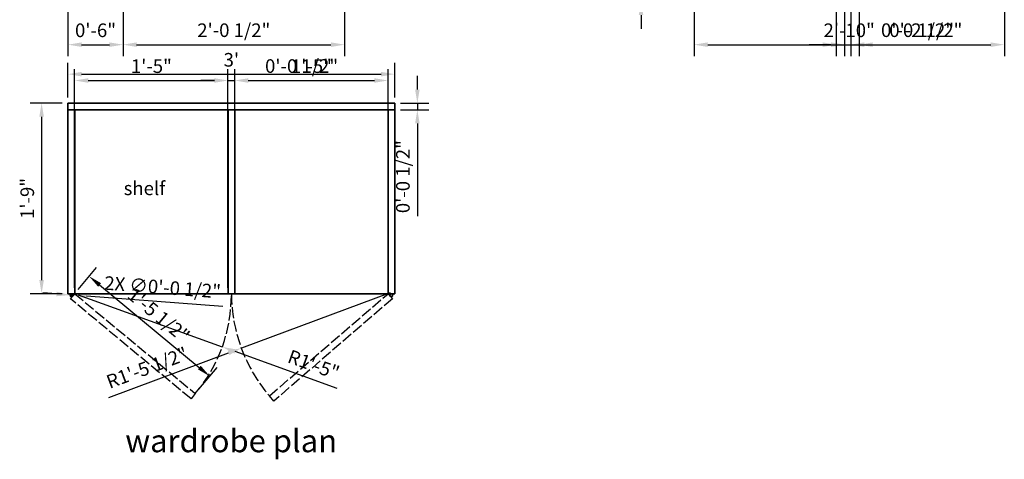
# Model space of a CAD drawing. Units: inches. Extents: x 1145 to 1264, y 2632 to 2775.
# Tile 1 of 2: x 1149 to 1257, y 2632 to 2681. Entities that reach past the tile are written whole.
import ezdxf

# ---------------------------------------------------------------- set-up
doc = ezdxf.new("R2010")
doc.units = ezdxf.units.IN
doc.linetypes.add('ACAD_ISO02W100', pattern=[15, 12, -3])
for name, color, linetype, lineweight in [('A-ANNO-DIMS', 2, 'Continuous', 18), ('A-ANNO-TEXT', 3, 'Continuous', 25), ('A-DOOR', 4, 'ACAD_ISO02W100', 25), ('A-FURN', 7, 'Continuous', 35)]:
    doc.layers.add(name, color=color, linetype=linetype, lineweight=lineweight)
doc.styles.get("Standard").update_dxf_attribs({"font": 'arial.ttf'})
doc.dimstyles.new('ISO-25', dxfattribs={"dimtxt": 1.5, "dimasz": 1.5, "dimexe": 1.25, "dimexo": 0.625, "dimtad": 1, "dimlunit": 3, "dimtxsty": 'Standard', "dimcen": 2.5, "dimadec": 0, "dimazin": 0, "dimtfac": 1, "dimtmove": 0, "dimatfit": 3, "dimfxl": 1, "dimarcsym": 0})

# ---------------------------------------------------------------- blocks, each defined once
blk = doc.blocks.new('*D1')
at = {"layer": 'A-ANNO-DIMS', "color": 0, "lineweight": -2, "transparency": 16777216}
for p, q in [((1153.92, 2671.95), (1153.92, 2675.76)), ((1189.92, 2671.95), (1189.92, 2675.76)), ((1155.42, 2674.51), (1188.42, 2674.51))]:
    blk.add_line(p, q, dxfattribs=at)
at = {"layer": 'A-ANNO-DIMS', "color": 0, "lineweight": 100, "transparency": 16777216}
for points in [[(1155.42, 2674.76), (1155.42, 2674.26), (1153.92, 2674.51)], [(1188.42, 2674.76), (1188.42, 2674.26), (1189.92, 2674.51)]]:
    blk.add_solid(points, dxfattribs=at)
at = {"layer": 'Defpoints', "color": 0, "lineweight": 100, "transparency": 16777216}
for p in [(1189.92, 2674.51), (1153.92, 2671.32), (1189.92, 2671.32)]:
    blk.add_point(p, dxfattribs=at)
at = {"layer": 'A-ANNO-DIMS', "color": 0, "transparency": 16777216, "insert": (1171.92, 2675.9), "char_height": 1.5, "attachment_point": 5}
blk.add_mtext("3'", dxfattribs=at)
blk = doc.blocks.new('*D2')
at = {"layer": 'A-ANNO-DIMS', "color": 0, "lineweight": -2, "transparency": 16777216}
for p, q in [((1153.3, 2671.32), (1149.77, 2671.32)), ((1151.02, 2669.82), (1151.02, 2651.82)), ((1153.3, 2650.32), (1149.77, 2650.32))]:
    blk.add_line(p, q, dxfattribs=at)
at = {"layer": 'A-ANNO-DIMS', "color": 0, "lineweight": 100, "transparency": 16777216}
for points in [[(1150.77, 2669.82), (1151.27, 2669.82), (1151.02, 2671.32)], [(1150.77, 2651.82), (1151.27, 2651.82), (1151.02, 2650.32)]]:
    blk.add_solid(points, dxfattribs=at)
at = {"layer": 'Defpoints', "color": 0, "lineweight": 100, "transparency": 16777216}
for p in [(1153.92, 2671.32), (1151.02, 2650.32), (1153.92, 2650.32)]:
    blk.add_point(p, dxfattribs=at)
at = {"layer": 'A-ANNO-DIMS', "color": 0, "transparency": 16777216, "insert": (1149.63, 2660.82), "char_height": 1.5, "attachment_point": 5, "rotation": 90}
blk.add_mtext('1\'-9"', dxfattribs=at)
blk = doc.blocks.new('*D21')
at = {"layer": 'A-ANNO-DIMS', "color": 0, "lineweight": -2, "transparency": 16777216}
for p, q in [((1153.92, 2681.89), (1153.92, 2676.51)), ((1159.99, 2682.21), (1159.99, 2676.51)), ((1155.42, 2677.76), (1158.49, 2677.76))]:
    blk.add_line(p, q, dxfattribs=at)
at = {"layer": 'A-ANNO-DIMS', "color": 0, "lineweight": 100, "transparency": 16777216}
for points in [[(1155.42, 2678.01), (1155.42, 2677.51), (1153.92, 2677.76)], [(1158.49, 2678.01), (1158.49, 2677.51), (1159.99, 2677.76)]]:
    blk.add_solid(points, dxfattribs=at)
at = {"layer": 'Defpoints', "color": 0, "lineweight": 100, "transparency": 16777216}
for p in [(1153.92, 2682.52), (1159.99, 2682.84), (1159.99, 2677.76)]:
    blk.add_point(p, dxfattribs=at)
at = {"layer": 'A-ANNO-DIMS', "color": 0, "transparency": 16777216, "insert": (1156.96, 2679.15), "char_height": 1.5, "attachment_point": 5}
blk.add_mtext('0\'-6"', dxfattribs=at)
blk = doc.blocks.new('*D22')
at = {"layer": 'A-ANNO-DIMS', "color": 0, "lineweight": -2, "transparency": 16777216}
for p, q in [((1159.99, 2682.21), (1159.99, 2676.51)), ((1184.39, 2682.21), (1184.39, 2676.51)), ((1161.49, 2677.76), (1182.89, 2677.76))]:
    blk.add_line(p, q, dxfattribs=at)
at = {"layer": 'A-ANNO-DIMS', "color": 0, "lineweight": 100, "transparency": 16777216}
for points in [[(1161.49, 2678.01), (1161.49, 2677.51), (1159.99, 2677.76)], [(1182.89, 2678.01), (1182.89, 2677.51), (1184.39, 2677.76)]]:
    blk.add_solid(points, dxfattribs=at)
at = {"layer": 'Defpoints', "color": 0, "lineweight": 100, "transparency": 16777216}
for p in [(1159.99, 2682.84), (1184.39, 2682.84), (1184.39, 2677.76)]:
    blk.add_point(p, dxfattribs=at)
at = {"layer": 'A-ANNO-DIMS', "color": 0, "transparency": 16777216, "insert": (1172.19, 2679.16), "char_height": 1.5, "attachment_point": 5}
blk.add_mtext('2\'-0 1/2"', dxfattribs=at)
blk = doc.blocks.new('*D26')
at = {"layer": 'A-ANNO-DIMS', "color": 0, "lineweight": -2, "transparency": 16777216}
for p, q in [((1238.56, 2720.63), (1238.56, 2676.51)), ((1241.06, 2720.63), (1241.06, 2676.51)), ((1237.06, 2677.76), (1235.56, 2677.76)), ((1238.56, 2677.76), (1241.06, 2677.76)), ((1242.56, 2677.76), (1252.79, 2677.76))]:
    blk.add_line(p, q, dxfattribs=at)
at = {"layer": 'A-ANNO-DIMS', "color": 0, "lineweight": 100, "transparency": 16777216}
for points in [[(1237.06, 2678.01), (1237.06, 2677.51), (1238.56, 2677.76)], [(1242.56, 2678.01), (1242.56, 2677.51), (1241.06, 2677.76)]]:
    blk.add_solid(points, dxfattribs=at)
at = {"layer": 'Defpoints', "color": 0, "lineweight": 100, "transparency": 16777216}
for p in [(1238.56, 2721.26), (1241.06, 2721.26), (1241.06, 2677.76)]:
    blk.add_point(p, dxfattribs=at)
at = {"layer": 'A-ANNO-DIMS', "color": 0, "transparency": 16777216, "insert": (1248.42, 2679.16), "char_height": 1.5, "attachment_point": 5}
blk.add_mtext('0\'-2 1/2"', dxfattribs=at)
blk = doc.blocks.new('*D28')
at = {"layer": 'A-ANNO-DIMS', "color": 0, "lineweight": -2, "transparency": 16777216}
for p, q in [((1239.47, 2760.15), (1239.47, 2676.51)), ((1240.15, 2760.15), (1240.15, 2676.51)), ((1237.97, 2677.76), (1236.47, 2677.76)), ((1239.47, 2677.76), (1240.15, 2677.76)), ((1241.65, 2677.76), (1251.88, 2677.76))]:
    blk.add_line(p, q, dxfattribs=at)
at = {"layer": 'A-ANNO-DIMS', "color": 0, "lineweight": 100, "transparency": 16777216}
for points in [[(1237.97, 2678.01), (1237.97, 2677.51), (1239.47, 2677.76)], [(1241.65, 2678.01), (1241.65, 2677.51), (1240.15, 2677.76)]]:
    blk.add_solid(points, dxfattribs=at)
at = {"layer": 'Defpoints', "color": 0, "lineweight": 100, "transparency": 16777216}
for p in [(1239.47, 2760.78), (1240.15, 2760.78), (1240.15, 2677.76)]:
    blk.add_point(p, dxfattribs=at)
at = {"layer": 'A-ANNO-DIMS', "color": 0, "transparency": 16777216, "insert": (1247.51, 2679.16), "char_height": 1.5, "attachment_point": 5}
blk.add_mtext('0\'-0 1/2"', dxfattribs=at)
blk = doc.blocks.new('*D29')
at = {"layer": 'A-ANNO-DIMS', "color": 0, "lineweight": -2, "transparency": 16777216}
for p, q in [((1222.89, 2683.39), (1222.89, 2676.51)), ((1257.07, 2683.39), (1257.07, 2676.51)), ((1224.39, 2677.76), (1255.57, 2677.76))]:
    blk.add_line(p, q, dxfattribs=at)
at = {"layer": 'A-ANNO-DIMS', "color": 0, "lineweight": 100, "transparency": 16777216}
for points in [[(1224.39, 2678.01), (1224.39, 2677.51), (1222.89, 2677.76)], [(1255.57, 2678.01), (1255.57, 2677.51), (1257.07, 2677.76)]]:
    blk.add_solid(points, dxfattribs=at)
at = {"layer": 'Defpoints', "color": 0, "lineweight": 100, "transparency": 16777216}
for p in [(1222.89, 2684.02), (1257.07, 2684.02), (1257.07, 2677.76)]:
    blk.add_point(p, dxfattribs=at)
at = {"layer": 'A-ANNO-DIMS', "color": 0, "transparency": 16777216, "insert": (1239.98, 2679.15), "char_height": 1.5, "attachment_point": 5}
blk.add_mtext('2\'-10"', dxfattribs=at)
blk = doc.blocks.new('*D31')
at = {"layer": 'A-ANNO-DIMS', "color": 0, "lineweight": -2, "transparency": 16777216}
for p, q in [((1217.05, 2685.52), (1217.05, 2695.75)), ((1221.92, 2684.02), (1215.8, 2684.02)), ((1217.05, 2682.52), (1217.05, 2684.02)), ((1221.92, 2682.52), (1215.8, 2682.52)), ((1217.05, 2681.02), (1217.05, 2679.52))]:
    blk.add_line(p, q, dxfattribs=at)
at = {"layer": 'A-ANNO-DIMS', "color": 0, "lineweight": 100, "transparency": 16777216}
for points in [[(1216.8, 2685.52), (1217.3, 2685.52), (1217.05, 2684.02)], [(1216.8, 2681.02), (1217.3, 2681.02), (1217.05, 2682.52)]]:
    blk.add_solid(points, dxfattribs=at)
at = {"layer": 'Defpoints', "color": 0, "lineweight": 100, "transparency": 16777216}
for p in [(1217.05, 2684.02), (1222.55, 2684.02), (1222.55, 2682.52)]:
    blk.add_point(p, dxfattribs=at)
at = {"layer": 'A-ANNO-DIMS', "color": 0, "transparency": 16777216, "insert": (1215.65, 2691.38), "char_height": 1.5, "attachment_point": 5, "rotation": 90}
blk.add_mtext('0\'-1 1/2"', dxfattribs=at)
blk = doc.blocks.new('*D33')
at = {"layer": 'A-ANNO-DIMS', "color": 0, "lineweight": -2, "transparency": 16777216}
for p, q in [((1192.41, 2672.82), (1192.41, 2674.32)), ((1190.55, 2671.32), (1193.66, 2671.32)), ((1190.55, 2670.58), (1193.66, 2670.58)), ((1192.41, 2671.32), (1192.41, 2670.58)), ((1192.41, 2669.08), (1192.41, 2658.85))]:
    blk.add_line(p, q, dxfattribs=at)
at = {"layer": 'A-ANNO-DIMS', "color": 0, "lineweight": 100, "transparency": 16777216}
for points in [[(1192.16, 2672.82), (1192.66, 2672.82), (1192.41, 2671.32)], [(1192.16, 2669.08), (1192.66, 2669.08), (1192.41, 2670.58)]]:
    blk.add_solid(points, dxfattribs=at)
at = {"layer": 'Defpoints', "color": 0, "lineweight": 100, "transparency": 16777216}
for p in [(1189.92, 2671.32), (1189.92, 2670.58), (1192.41, 2670.58)]:
    blk.add_point(p, dxfattribs=at)
at = {"layer": 'A-ANNO-DIMS', "color": 0, "transparency": 16777216, "insert": (1191.01, 2663.22), "char_height": 1.5, "attachment_point": 5, "rotation": 90}
blk.add_mtext('0\'-0 1/2"', dxfattribs=at)
blk = doc.blocks.new('*D34')
at = {"layer": 'A-ANNO-DIMS', "color": 0, "lineweight": -2, "transparency": 16777216}
for p, q in [((1154.66, 2650.95), (1154.66, 2675.06)), ((1171.55, 2650.95), (1171.55, 2675.06)), ((1156.16, 2673.81), (1170.05, 2673.81))]:
    blk.add_line(p, q, dxfattribs=at)
at = {"layer": 'A-ANNO-DIMS', "color": 0, "lineweight": 100, "transparency": 16777216}
for points in [[(1156.16, 2674.06), (1156.16, 2673.56), (1154.66, 2673.81)], [(1170.05, 2674.06), (1170.05, 2673.56), (1171.55, 2673.81)]]:
    blk.add_solid(points, dxfattribs=at)
at = {"layer": 'Defpoints', "color": 0, "lineweight": 100, "transparency": 16777216}
for p in [(1171.55, 2673.81), (1154.66, 2650.32), (1171.55, 2650.32)]:
    blk.add_point(p, dxfattribs=at)
at = {"layer": 'A-ANNO-DIMS', "color": 0, "transparency": 16777216, "insert": (1163.11, 2675.2), "char_height": 1.5, "attachment_point": 5}
blk.add_mtext('1\'-5"', dxfattribs=at)
blk = doc.blocks.new('*D35')
at = {"layer": 'A-ANNO-DIMS', "color": 0, "lineweight": -2, "transparency": 16777216}
for p, q in [((1172.29, 2650.95), (1172.29, 2675.06)), ((1189.18, 2650.95), (1189.18, 2675.06)), ((1173.79, 2673.81), (1187.68, 2673.81))]:
    blk.add_line(p, q, dxfattribs=at)
at = {"layer": 'A-ANNO-DIMS', "color": 0, "lineweight": 100, "transparency": 16777216}
for points in [[(1173.79, 2674.06), (1173.79, 2673.56), (1172.29, 2673.81)], [(1187.68, 2674.06), (1187.68, 2673.56), (1189.18, 2673.81)]]:
    blk.add_solid(points, dxfattribs=at)
at = {"layer": 'Defpoints', "color": 0, "lineweight": 100, "transparency": 16777216}
for p in [(1189.18, 2673.81), (1172.29, 2650.32), (1189.18, 2650.32)]:
    blk.add_point(p, dxfattribs=at)
at = {"layer": 'A-ANNO-DIMS', "color": 0, "transparency": 16777216, "insert": (1180.74, 2675.2), "char_height": 1.5, "attachment_point": 5}
blk.add_mtext('1\'-5"', dxfattribs=at)
blk = doc.blocks.new('*D36')
at = {"layer": 'A-ANNO-DIMS', "color": 0, "lineweight": -2, "transparency": 16777216}
for p, q in [((1171.55, 2671.21), (1171.55, 2675.06)), ((1172.29, 2671.21), (1172.29, 2675.06)), ((1170.05, 2673.81), (1168.55, 2673.81)), ((1171.55, 2673.81), (1172.29, 2673.81)), ((1173.79, 2673.81), (1184.03, 2673.81))]:
    blk.add_line(p, q, dxfattribs=at)
at = {"layer": 'A-ANNO-DIMS', "color": 0, "lineweight": 100, "transparency": 16777216}
for points in [[(1170.05, 2674.06), (1170.05, 2673.56), (1171.55, 2673.81)], [(1173.79, 2674.06), (1173.79, 2673.56), (1172.29, 2673.81)]]:
    blk.add_solid(points, dxfattribs=at)
at = {"layer": 'Defpoints', "color": 0, "lineweight": 100, "transparency": 16777216}
for p in [(1172.29, 2673.81), (1171.55, 2670.58), (1172.29, 2670.58)]:
    blk.add_point(p, dxfattribs=at)
at = {"layer": 'A-ANNO-DIMS', "color": 0, "transparency": 16777216, "insert": (1179.66, 2675.21), "char_height": 1.5, "attachment_point": 5}
blk.add_mtext('0\'-0 1/2"', dxfattribs=at)
blk = doc.blocks.new('*D37')
at = {"layer": 'A-ANNO-DIMS', "color": 0, "lineweight": -2, "transparency": 16777216}
for p, q in [((1155.06, 2650.8), (1157.05, 2653.2)), ((1157.41, 2651.28), (1168.39, 2642.18)), ((1168.35, 2639.79), (1170.34, 2642.19))]:
    blk.add_line(p, q, dxfattribs=at)
at = {"layer": 'A-ANNO-DIMS', "color": 0, "lineweight": 100, "transparency": 16777216}
for points in [[(1157.57, 2651.48), (1157.25, 2651.09), (1156.25, 2652.24)], [(1168.55, 2642.38), (1168.23, 2641.99), (1169.54, 2641.23)]]:
    blk.add_solid(points, dxfattribs=at)
at = {"layer": 'Defpoints', "color": 0, "lineweight": 100, "transparency": 16777216}
for p in [(1154.66, 2650.32), (1169.54, 2641.23), (1167.95, 2639.31)]:
    blk.add_point(p, dxfattribs=at)
at = {"layer": 'A-ANNO-DIMS', "color": 0, "transparency": 16777216, "insert": (1163.79, 2647.81), "char_height": 1.5, "attachment_point": 5, "rotation": 320.3478}
blk.add_mtext('1\'-5 1/2"', dxfattribs=at)
blk = doc.blocks.new('*D39')
at = {"layer": 'A-ANNO-DIMS', "color": 0, "lineweight": -2, "transparency": 16777216}
for p, q in [((1189.4, 2650.4), (1173.02, 2644.32)), ((1158.42, 2638.89), (1171.61, 2643.79))]:
    blk.add_line(p, q, dxfattribs=at)
at = {"layer": 'A-ANNO-DIMS', "color": 0, "lineweight": 100, "transparency": 16777216}
blk.add_solid([(1171.52, 2644.03), (1171.7, 2643.56), (1173.02, 2644.32)], dxfattribs=at)
at = {"layer": 'Defpoints', "color": 0, "lineweight": 100, "transparency": 16777216}
for p in [(1189.4, 2650.4), (1173.02, 2644.32)]:
    blk.add_point(p, dxfattribs=at)
at = {"layer": 'A-ANNO-DIMS', "color": 0, "transparency": 16777216, "insert": (1162.7, 2641.98), "char_height": 1.5, "attachment_point": 5, "rotation": 20.3856}
blk.add_mtext('R1\'-5 1/2"', dxfattribs=at)
blk = doc.blocks.new('*D40')
at = {"layer": 'A-ANNO-DIMS', "color": 0, "lineweight": -2, "transparency": 16777216}
for p, q in [((1155.04, 2650.19), (1170.92, 2644.46)), ((1183.59, 2639.89), (1172.33, 2643.95))]:
    blk.add_line(p, q, dxfattribs=at)
at = {"layer": 'A-ANNO-DIMS', "color": 0, "lineweight": 100, "transparency": 16777216}
blk.add_solid([(1172.42, 2644.19), (1172.25, 2643.72), (1170.92, 2644.46)], dxfattribs=at)
at = {"layer": 'Defpoints', "color": 0, "lineweight": 100, "transparency": 16777216}
for p in [(1155.04, 2650.19), (1170.92, 2644.46)]:
    blk.add_point(p, dxfattribs=at)
at = {"layer": 'A-ANNO-DIMS', "color": 0, "transparency": 16777216, "insert": (1180.92, 2642.33), "char_height": 1.5, "attachment_point": 5, "rotation": 340.173}
blk.add_mtext('R1\'-5"', dxfattribs=at)
blk = doc.blocks.new('*D41')
at = {"layer": 'A-ANNO-DIMS', "color": 0, "lineweight": -2, "transparency": 16777216}
for p, q in [((1152.67, 2650.29), (1151.17, 2650.4)), ((1154.16, 2650.17), (1154.48, 2650.15)), ((1170.97, 2648.9), (1155.98, 2650.04))]:
    blk.add_line(p, q, dxfattribs=at)
at = {"layer": 'A-ANNO-DIMS', "color": 0, "lineweight": 100, "transparency": 16777216}
for points in [[(1152.69, 2650.54), (1152.65, 2650.04), (1154.16, 2650.17)], [(1156, 2650.29), (1155.96, 2649.79), (1154.48, 2650.15)]]:
    blk.add_solid(points, dxfattribs=at)
at = {"layer": 'Defpoints', "color": 0, "lineweight": 100, "transparency": 16777216}
for p in [(1154.16, 2650.17), (1154.48, 2650.15)]:
    blk.add_point(p, dxfattribs=at)
at = {"layer": 'A-ANNO-DIMS', "color": 0, "transparency": 16777216, "insert": (1164.33, 2650.84), "char_height": 1.5, "attachment_point": 5, "rotation": 355.6561}
blk.add_mtext('2X ∅0\'-0 1/2"', dxfattribs=at)

msp = doc.modelspace()

# ---------------------------------------------------------------- linework, layer by layer
at = {"layer": 'A-DOOR'}
msp.add_line((1171.923, 2670.583), (1172.663, 2670.583), dxfattribs=at)
at = {"layer": 'A-DOOR', "ltscale": 0.1}
for points in [[(1154.663, 2650.323), (1167.952, 2639.309), (1167.48, 2638.74), (1154.19, 2649.754)], [(1189.666, 2649.763), (1176.594, 2638.492), (1176.111, 2639.053), (1189.183, 2650.323)]]:
    msp.add_lwpolyline(points, close=True, dxfattribs=at)
for centre, radius, start, end in [((1155.039, 2650.188), 16.884, 319.88758, 0.46025), ((1189.395, 2650.402), 17.473, 180.25878, 220.50974)]:
    msp.add_arc(centre, radius, start, end, dxfattribs=at)
at = {"layer": 'A-FURN'}
for p, q in [((1153.923, 2671.323), (1189.923, 2671.323)), ((1153.923, 2650.323), (1153.923, 2671.323)), ((1153.923, 2670.583), (1189.923, 2670.583)), ((1154.663, 2650.323), (1154.663, 2670.583)), ((1171.553, 2670.583), (1171.553, 2650.323)), ((1172.293, 2670.583), (1172.293, 2650.323)), ((1189.183, 2670.583), (1189.183, 2650.323)), ((1189.923, 2671.323), (1189.923, 2650.323)), ((1189.923, 2650.323), (1153.923, 2650.323)), ((1154.663, 2650.323), (1189.183, 2650.323))]:
    msp.add_line(p, q, dxfattribs=at)
for centre in [(1154.324, 2650.162), (1189.531, 2650.163)]:
    msp.add_circle(centre, 0.16, dxfattribs=at)

# ---------------------------------------------------------------- texts
at = {"layer": 'A-ANNO-TEXT', "ltscale": 0.5, "insert": (1160.058, 2662.683), "char_height": 1.5, "attachment_point": 1}
msp.add_mtext_dynamic_manual_height_columns('shelf', width=12.71278, gutter_width=12.5, heights=[0], dxfattribs=at)
at = {"layer": 'A-ANNO-TEXT', "insert": (1160.237, 2635.354), "char_height": 2.5, "attachment_point": 1}
msp.add_mtext_dynamic_manual_height_columns('wardrobe plan', width=36.11329, gutter_width=12.5, heights=[0], dxfattribs=at)

# ---------------------------------------------------------------- dimensions: what is measured, and where the dimension line sits
at = {"layer": 'A-ANNO-DIMS'}
for base, p1, p2, override, picture, middle in [((1240.146, 2677.758), (1239.466, 2760.778), (1240.146, 2760.778), {"dimdec": 1, "dimlfac": 1, "dimrnd": 0, "dimzin": 1, "dimdsep": 46, "dimlunit": 4, "dimfrac": 2}, '*D28', (1247.512, 2679.159)), ((1241.056, 2677.758), (1238.556, 2721.258), (1241.056, 2721.258), {"dimdec": 1, "dimlfac": 1, "dimrnd": 0, "dimzin": 1, "dimdsep": 46, "dimlunit": 4, "dimfrac": 2}, '*D26', (1248.422, 2679.159)), ((1257.066, 2677.758), (1222.886, 2684.018), (1257.066, 2684.018), {"dimdec": 1, "dimlfac": 1, "dimrnd": 0, "dimzin": 1, "dimdsep": 46, "dimlunit": 4, "dimfrac": 2}, '*D29', (1239.976, 2679.149)), ((1159.991, 2677.758), (1153.923, 2682.518), (1159.991, 2682.836), {"dimdec": 1, "dimlfac": 1, "dimrnd": 0, "dimzin": 1, "dimdsep": 46, "dimlunit": 4, "dimfrac": 2}, '*D21', (1156.957, 2679.149)), ((1184.387, 2677.758), (1159.991, 2682.836), (1184.387, 2682.836), {"dimdec": 1, "dimlfac": 1, "dimrnd": 0, "dimzin": 1, "dimdsep": 46, "dimlunit": 4, "dimfrac": 2}, '*D22', (1172.189, 2679.159)), ((1189.923, 2674.513), (1153.923, 2671.323), (1189.923, 2671.323), {"dimclrd": 0, "dimclre": 0, "dimclrt": 0}, '*D1', (1171.923, 2675.905)), ((1172.293, 2673.813), (1171.553, 2670.583), (1172.293, 2670.583), {"dimdec": 1, "dimlfac": 1, "dimrnd": 0, "dimzin": 1, "dimdsep": 46, "dimlunit": 4, "dimfrac": 2}, '*D36', (1179.659, 2675.214)), ((1171.553, 2673.813), (1154.663, 2650.323), (1171.553, 2650.323), {"dimdec": 1, "dimlfac": 1, "dimrnd": 0, "dimzin": 1, "dimdsep": 46, "dimlunit": 4, "dimfrac": 2}, '*D34', (1163.108, 2675.204)), ((1189.183, 2673.813), (1172.293, 2650.323), (1189.183, 2650.323), {"dimdec": 1, "dimlfac": 1, "dimrnd": 0, "dimzin": 1, "dimdsep": 46, "dimlunit": 4, "dimfrac": 2}, '*D35', (1180.738, 2675.204))]:
    dim = msp.add_linear_dim(base=base, p1=p1, p2=p2, dimstyle='ISO-25', override=override, dxfattribs=at)
    dim.commit()
    dim.dimension.update_dxf_attribs({"geometry": picture, "text_midpoint": middle})
for base, p1, p2, angle, override, picture, middle in [((1217.046, 2684.018), (1222.546, 2682.518), (1222.546, 2684.018), 90, {"dimdec": 1, "dimlfac": 1, "dimrnd": 0, "dimzin": 1, "dimdsep": 46, "dimlunit": 4, "dimfrac": 2}, '*D31', (1215.645, 2691.385)), ((1192.413, 2670.583), (1189.923, 2671.323), (1189.923, 2670.583), 90, {"dimdec": 1, "dimlfac": 1, "dimrnd": 0, "dimzin": 1, "dimdsep": 46, "dimlunit": 4, "dimfrac": 2}, '*D33', (1191.012, 2663.217)), ((1151.018, 2650.323), (1153.923, 2671.323), (1153.923, 2650.323), 90, {"dimclrd": 0, "dimclre": 0, "dimclrt": 0}, '*D2', (1149.627, 2660.823)), ((1169.541, 2641.226), (1154.663, 2650.323), (1167.952, 2639.309), 320.34783, {"dimdec": 1, "dimlfac": 1, "dimrnd": 0, "dimzin": 1, "dimdsep": 46, "dimlunit": 4, "dimfrac": 2}, '*D37', (1163.79, 2647.812))]:
    dim = msp.add_linear_dim(base=base, p1=p1, p2=p2, angle=angle, dimstyle='ISO-25', override=override, dxfattribs=at)
    dim.commit()
    dim.dimension.update_dxf_attribs({"geometry": picture, "text_midpoint": middle})
dim = msp.add_diameter_dim_2p(p1=(1154.165, 2650.174), p2=(1154.484, 2650.15), text='2X <>', dimstyle='ISO-25', override={"dimdec": 1, "dimlfac": 1, "dimrnd": 0, "dimzin": 1, "dimdsep": 46, "dimlunit": 4, "dimfrac": 2}, dxfattribs=at)
dim.commit()
dim.dimension.update_dxf_attribs({"geometry": '*D41', "text_midpoint": (1164.222, 2649.41)})
for center, mpoint, picture, middle in [((1155.039, 2650.188), (1170.922, 2644.461), '*D40', (1180.452, 2641.025)), ((1189.395, 2650.402), (1173.017, 2644.316), '*D39', (1163.19, 2640.664))]:
    dim = msp.add_radius_dim(center=center, mpoint=mpoint, dimstyle='ISO-25', override={"dimdec": 1, "dimlfac": 1, "dimrnd": 0, "dimzin": 1, "dimdsep": 46, "dimlunit": 4, "dimfrac": 2}, dxfattribs=at)
    dim.commit()
    dim.dimension.update_dxf_attribs({"geometry": picture, "text_midpoint": middle, "dimtype": 164})

doc.saveas('drawing.dxf')
